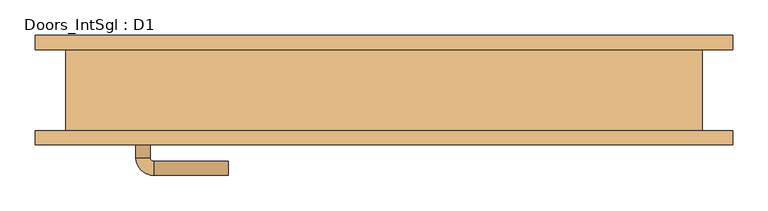
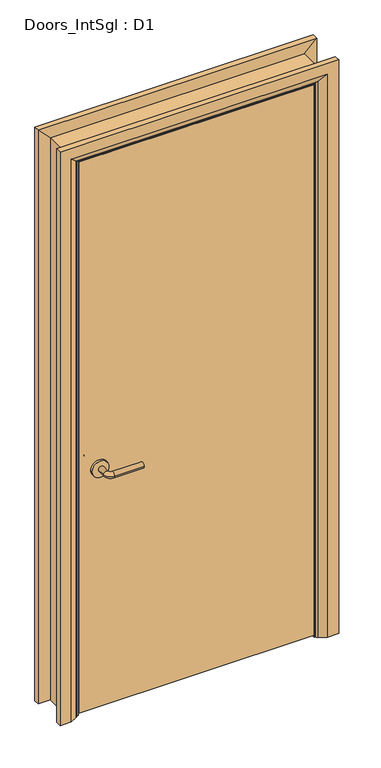
"""IFC4 building model written with IfcOpenShell, lengths in millimetres: door geometry, Doors_IntSgl : D1."""

from ifc_helpers import new_model, si_unit, point, frame, frame_2d, origin, place, context, project, spatial, polyline, circle_curve, ellipse_curve, trimmed, segment, composite_curve, outline, extrude, faceted_brep, source, transform, mapped, element, save
from ifc_brep_helpers import plane_surface, cylinder_surface, revolved_surface, advanced_brep


def doors_intsgl_d1_d2de26da(model_context):
    return source(origin(), model_context, "Body", "SolidModel", [
        advanced_brep(
        [(-350.2, -11.15, 900.0), (-330.2, -11.15, 900.0), (-350.2, 18.85, 900.0), (-330.2, 18.85, 900.0), (-325.2, 23.85, 900.0), (-325.2, 43.85, 900.0), (-220.2, 43.85, 900.0), (-220.2, 23.85, 900.0)],
        [
            (0, 1, circle_curve(frame((-340.2, -11.15, 900.0), z_axis=(0.0, -1.0, 0.0), x_axis=(1.0, 0.0, 0.0)), 10.0)),
            (1, 0, circle_curve(frame((-340.2, -11.15, 900.0), z_axis=(0.0, -1.0, 0.0), x_axis=(1.0, 0.0, 0.0)), 10.0)),
            (0, 2),
            (2, 3, circle_curve(frame((-340.2, 18.85, 900.0), z_axis=(0.0, -1.0, 0.0), x_axis=(1.0, 0.0, 0.0)), 10.0)),
            (3, 1),
            (3, 2, circle_curve(frame((-340.2, 18.85, 900.0), z_axis=(0.0, -1.0, 0.0), x_axis=(1.0, 0.0, 0.0)), 10.0)),
            (4, 3, circle_curve(frame((-325.2, 18.85, 900.0), z_axis=(0.0, 0.0, 1.0), x_axis=(-1.0, 0.0, 0.0)), 5.0)),
            (2, 5, circle_curve(frame((-325.2, 18.85, 900.0), z_axis=(0.0, 0.0, -1.0), x_axis=(-1.0, 0.0, 0.0)), 25.0)),
            (5, 4, circle_curve(frame((-325.2, 33.85, 900.0), z_axis=(-1.0, 0.0, 0.0), x_axis=(0.0, -1.0, 0.0)), 10.0)),
            (4, 5, circle_curve(frame((-325.2, 33.85, 900.0), z_axis=(-1.0, 0.0, 0.0), x_axis=(0.0, -1.0, 0.0)), 10.0)),
            (6, 7, circle_curve(frame((-220.2, 33.85, 900.0), z_axis=(1.0, 0.0, 0.0), x_axis=(0.0, -1.0, 0.0)), 10.0)),
            (7, 6, circle_curve(frame((-220.2, 33.85, 900.0), z_axis=(1.0, 0.0, 0.0), x_axis=(0.0, -1.0, 0.0)), 10.0)),
            (5, 6),
            (7, 4),
        ],
        [
            plane_surface(frame((-340.2, -11.15, 900.0), z_axis=(0.0, -1.0, 0.0), x_axis=(0.0, 0.0, 1.0))),
            cylinder_surface(frame((-340.2, -11.15, 900.0), z_axis=(0.0, -1.0, 0.0), x_axis=(1.0, 0.0, 0.0)), 10.0),
            revolved_surface(trimmed(ellipse_curve(frame((-340.2, 18.85, 900.0), z_axis=(0.0, -1.0, 0.0), x_axis=(1.0, 0.0, 0.0)), 10.0, 10.0), [point((-350.2, 18.85, 900.0))], [point((-330.2, 18.85, 900.0))], True, "CARTESIAN"), (-325.2, 18.85, 900.0), (0.0, 0.0, -1.0)),
            revolved_surface(trimmed(ellipse_curve(frame((-340.2, 18.85, 900.0), z_axis=(0.0, -1.0, 0.0), x_axis=(1.0, 0.0, 0.0)), 10.0, 10.0), [point((-330.2, 18.85, 900.0))], [point((-350.2, 18.85, 900.0))], True, "CARTESIAN"), (-325.2, 18.85, 900.0), (0.0, 0.0, -1.0)),
            plane_surface(frame((-220.2, 33.85, 900.0), z_axis=(1.0, 0.0, 0.0), x_axis=(0.0, 0.0, 1.0))),
            cylinder_surface(frame((-325.2, 33.85, 900.0), z_axis=(-1.0, 0.0, 0.0), x_axis=(0.0, -1.0, 0.0)), 10.0),
        ],
        [
            (0, [[1, 2]]),
            (1, [[-1, 3, 4, 5]]),
            (1, [[-2, -5, 6, -3]]),
            (2, [[7, -4, 8, 9]]),
            (3, [[-8, -6, -7, 10]]),
            (4, [[11, 12]]),
            (5, [[-9, 13, -12, 14]]),
            (5, [[-10, -14, -11, -13]]),
        ],
    ),
        extrude(outline(composite_curve([segment(trimmed(circle_curve(frame_2d((900.0, -342.7)), 30.0), [point((900.0, -372.7))], [point((900.0, -312.7))], False, "CARTESIAN"), True, "CONTINUOUS"), segment(trimmed(circle_curve(frame_2d((900.0, -342.7)), 30.0), [point((900.0, -312.7))], [point((900.0, -372.7))], False, "CARTESIAN"), True, "CONTINUOUS")], self_intersect=False)), frame((0.0, -19.15, 0.0), z_axis=(0.0, 1.0, 0.0), x_axis=(0.0, 0.0, 1.0)), (0.0, 0.0, 1.0), 8.0),
        advanced_brep(
        [(-350.2, -65.15, 900.0), (-330.2, -65.15, 900.0), (-330.2, -95.15, 900.0), (-350.2, -95.15, 900.0), (-325.2, -100.15, 900.0), (-325.2, -120.15, 900.0), (-220.2, -120.15, 900.0), (-220.2, -100.15, 900.0)],
        [
            (0, 1, circle_curve(frame((-340.2, -65.15, 900.0), z_axis=(0.0, 1.0, 0.0), x_axis=(1.0, 0.0, 0.0)), 10.0)),
            (1, 0, circle_curve(frame((-340.2, -65.15, 900.0), z_axis=(0.0, 1.0, 0.0), x_axis=(1.0, 0.0, 0.0)), 10.0)),
            (1, 2),
            (2, 3, circle_curve(frame((-340.2, -95.15, 900.0), z_axis=(0.0, 1.0, 0.0), x_axis=(1.0, 0.0, 0.0)), 10.0)),
            (3, 0),
            (3, 2, circle_curve(frame((-340.2, -95.15, 900.0), z_axis=(0.0, 1.0, 0.0), x_axis=(1.0, 0.0, 0.0)), 10.0)),
            (4, 5, circle_curve(frame((-325.2, -110.15, 900.0), z_axis=(-1.0, 0.0, 0.0), x_axis=(0.0, 1.0, 0.0)), 10.0)),
            (5, 3, circle_curve(frame((-325.2, -95.15, 900.0), z_axis=(0.0, 0.0, -1.0), x_axis=(-1.0, 0.0, 0.0)), 25.0)),
            (2, 4, circle_curve(frame((-325.2, -95.15, 900.0), z_axis=(0.0, 0.0, 1.0), x_axis=(-1.0, 0.0, 0.0)), 5.0)),
            (5, 4, circle_curve(frame((-325.2, -110.15, 900.0), z_axis=(-1.0, 0.0, 0.0), x_axis=(0.0, 1.0, 0.0)), 10.0)),
            (6, 7, circle_curve(frame((-220.2, -110.15, 900.0), z_axis=(1.0, 0.0, 0.0), x_axis=(0.0, 1.0, 0.0)), 10.0)),
            (7, 6, circle_curve(frame((-220.2, -110.15, 900.0), z_axis=(1.0, 0.0, 0.0), x_axis=(0.0, 1.0, 0.0)), 10.0)),
            (4, 7),
            (6, 5),
        ],
        [
            plane_surface(frame((-340.2, -65.15, 900.0), z_axis=(0.0, 1.0, 0.0), x_axis=(0.0, 0.0, 1.0))),
            cylinder_surface(frame((-340.2, -65.15, 900.0), z_axis=(0.0, 1.0, 0.0), x_axis=(1.0, 0.0, 0.0)), 10.0),
            revolved_surface(trimmed(ellipse_curve(frame((-340.2, -95.15, 900.0), z_axis=(0.0, -1.0, 0.0), x_axis=(1.0, 0.0, 0.0)), 10.0, 10.0), [point((-350.2, -95.15, 900.0))], [point((-330.2, -95.15, 900.0))], True, "CARTESIAN"), (-325.2, -95.15, 900.0), (0.0, 0.0, -1.0)),
            revolved_surface(trimmed(ellipse_curve(frame((-340.2, -95.15, 900.0), z_axis=(0.0, -1.0, 0.0), x_axis=(1.0, 0.0, 0.0)), 10.0, 10.0), [point((-330.2, -95.15, 900.0))], [point((-350.2, -95.15, 900.0))], True, "CARTESIAN"), (-325.2, -95.15, 900.0), (0.0, 0.0, -1.0)),
            plane_surface(frame((-220.2, -110.15, 900.0), z_axis=(1.0, 0.0, 0.0), x_axis=(0.0, 0.0, 1.0))),
            cylinder_surface(frame((-325.2, -110.15, 900.0), z_axis=(-1.0, 0.0, 0.0), x_axis=(0.0, 1.0, 0.0)), 10.0),
        ],
        [
            (0, [[1, 2]]),
            (1, [[3, 4, 5, -2]]),
            (1, [[-5, 6, -3, -1]]),
            (2, [[7, 8, -4, 9]]),
            (3, [[10, -9, -6, -8]]),
            (4, [[11, 12]]),
            (5, [[13, -11, 14, -7]]),
            (5, [[-14, -12, -13, -10]]),
        ],
    ),
        extrude(outline(composite_curve([segment(trimmed(circle_curve(frame_2d((900.0, -342.7)), 30.0), [point((900.0, -372.7))], [point((900.0, -312.7))], False, "CARTESIAN"), True, "CONTINUOUS"), segment(trimmed(circle_curve(frame_2d((900.0, -342.7)), 30.0), [point((900.0, -312.7))], [point((900.0, -372.7))], False, "CARTESIAN"), True, "CONTINUOUS")], self_intersect=False)), frame((0.0, -65.15, 0.0), z_axis=(0.0, 1.0, 0.0), x_axis=(0.0, 0.0, 1.0)), (0.0, 0.0, 1.0), 8.0),
        extrude(outline(polyline([(415.2, -19.15), (415.2, -57.15), (-415.2, -57.15), (-415.2, -19.15), (415.2, -19.15)])), frame((0.0, 0.0, 8.0), z_axis=(0.0, 0.0, 1.0), x_axis=(1.0, 0.0, 0.0)), (0.0, 0.0, 1.0), 2060.0),
        advanced_brep(
        [(492.2, -77.15, 0.0), (452.2, -77.15, 0.0), (426.2, -63.15, 0.0), (422.2, -57.15, 0.0), (492.2, -57.15, 0.0), (492.2, -57.15, 2145.0), (492.2, -77.15, 2145.0), (422.2, -57.15, 2075.0), (-422.2, -57.15, 2075.0), (-422.2, -57.15, 0.0), (-492.2, -57.15, 0.0), (-492.2, -57.15, 2145.0), (426.2, -63.15, 2079.0), (452.2, -77.15, 2105.0), (-492.2, -77.15, 2145.0), (-492.2, -77.15, 0.0), (-452.2, -77.15, 0.0), (-452.2, -77.15, 2105.0), (-426.2, -63.15, 0.0), (-426.2, -63.15, 2079.0)],
        [
            (0, 1),
            (1, 2),
            (2, 3, circle_curve(frame((430.2, -56.15, 0.0), z_axis=(0.0, 0.0, -1.0), x_axis=(1.0, 0.0, 0.0)), 8.0622577)),
            (3, 4),
            (4, 0),
            (4, 5),
            (5, 6),
            (6, 0),
            (3, 7),
            (7, 8),
            (8, 9),
            (9, 10),
            (10, 11),
            (11, 5),
            (2, 12),
            (12, 7, ellipse_curve(frame((430.2, -56.15, 2083.0), z_axis=(0.7071067811865475, 0.0, -0.7071067811865475), x_axis=(-0.7071067811865474, 0.0, -0.7071067811865476)), 11.4017543, 8.0622577)),
            (1, 13),
            (13, 12),
            (6, 14),
            (14, 15),
            (15, 16),
            (16, 17),
            (17, 13),
            (10, 15),
            (14, 11),
            (9, 18, circle_curve(frame((-430.2, -56.15, 0.0), z_axis=(0.0, 0.0, -1.0), x_axis=(-1.0, 0.0, 0.0)), 8.0622577)),
            (18, 16),
            (19, 18),
            (8, 19, ellipse_curve(frame((-430.2, -56.15, 2083.0), z_axis=(-0.7071067811865475, 0.0, -0.7071067811865475), x_axis=(-0.7071067811865474, 0.0, 0.7071067811865476)), 11.4017543, 8.0622577)),
            (19, 17),
            (12, 19),
        ],
        [
            plane_surface(frame((422.2, -57.15, 0.0), z_axis=(0.0, 0.0, -1.0), x_axis=(0.0, 1.0, 0.0))),
            plane_surface(frame((492.2, -77.15, 0.0), z_axis=(1.0, 0.0, 0.0), x_axis=(0.0, 0.0, 1.0))),
            plane_surface(frame((492.2, -57.15, 0.0), z_axis=(0.0, 1.0, 0.0), x_axis=(0.0, 0.0, 1.0))),
            cylinder_surface(frame((430.2, -56.15, 0.0), z_axis=(0.0, 0.0, -1.0), x_axis=(1.0, 0.0, 0.0)), 8.0622577),
            plane_surface(frame((426.2, -63.15, 0.0), z_axis=(-0.4740998230350126, -0.880471099922178, 0.0), x_axis=(0.0, 0.0, 1.0))),
            plane_surface(frame((452.2, -77.15, 0.0), z_axis=(0.0, -1.0, 0.0), x_axis=(0.0, 0.0, 1.0))),
            plane_surface(frame((-492.2, -77.15, 2145.0), z_axis=(-1.0, 0.0, 0.0), x_axis=(0.0, 0.0, -1.0))),
            plane_surface(frame((-422.2, -57.15, 0.0), z_axis=(0.0, 0.0, -1.0), x_axis=(0.0, 1.0, 0.0))),
            cylinder_surface(frame((-430.2, -56.15, 2075.0), z_axis=(0.0, 0.0, 1.0), x_axis=(-1.0, 0.0, 0.0)), 8.0622577),
            plane_surface(frame((-426.2, -63.15, 2079.0), z_axis=(0.47409982303501824, -0.8804710999221749, 0.0), x_axis=(0.0, 0.0, -1.0))),
            plane_surface(frame((492.2, -77.15, 2145.0), z_axis=(0.0, 0.0, 1.0), x_axis=(-1.0, 0.0, 0.0))),
            cylinder_surface(frame((422.2, -56.15, 2083.0), z_axis=(1.0, 0.0, 0.0), x_axis=(0.0, 0.0, 1.0)), 8.0622577),
            plane_surface(frame((426.2, -63.15, 2079.0), z_axis=(0.0, -0.8804710999221764, -0.4740998230350154), x_axis=(-1.0, 0.0, 0.0))),
        ],
        [
            (0, [[1, 2, 3, 4, 5]]),
            (1, [[6, 7, 8, -5]]),
            (2, [[9, 10, 11, 12, 13, 14, -6, -4]]),
            (3, [[15, 16, -9, -3]]),
            (4, [[17, 18, -15, -2]]),
            (5, [[-8, 19, 20, 21, 22, 23, -17, -1]]),
            (6, [[-13, 24, -20, 25]]),
            (7, [[-24, -12, 26, 27, -21]]),
            (8, [[28, -26, -11, 29]]),
            (9, [[-22, -27, -28, 30]]),
            (10, [[-14, -25, -19, -7]]),
            (11, [[31, -29, -10, -16]]),
            (12, [[-23, -30, -31, -18]]),
        ],
    ),
        extrude(outline(polyline([(0.0, -398.2), (2051.0, -398.2), (2051.0, 398.2), (0.0, 398.2), (0.0, 417.2), (2070.0, 417.2), (2070.0, -417.2), (0.0, -417.2), (0.0, -398.2)])), frame((0.0, -17.15, 0.0), z_axis=(0.0, 1.0, 0.0), x_axis=(0.0, 0.0, 1.0)), (0.0, 0.0, 1.0), 32.0),
        advanced_brep(
        [(-492.2, 77.15, 0.0), (-452.2, 77.15, 0.0), (-426.2, 63.15, 0.0), (-422.2, 57.15, 0.0), (-492.2, 57.15, 0.0), (-492.2, 57.15, 2145.0), (-492.2, 77.15, 2145.0), (-422.2, 57.15, 2075.0), (-426.2, 63.15, 2079.0), (-452.2, 77.15, 2105.0), (492.2, 77.15, 0.0), (492.2, 57.15, 0.0), (422.2, 57.15, 0.0), (426.2, 63.15, 0.0), (452.2, 77.15, 0.0), (492.2, 77.15, 2145.0), (452.2, 77.15, 2105.0), (426.2, 63.15, 2079.0), (422.2, 57.15, 2075.0), (492.2, 57.15, 2145.0)],
        [
            (0, 1),
            (1, 2),
            (2, 3, circle_curve(frame((-430.2, 56.15, 0.0), z_axis=(0.0, 0.0, -1.0), x_axis=(-1.0, 0.0, 0.0)), 8.0622577)),
            (3, 4),
            (4, 0),
            (4, 5),
            (5, 6),
            (6, 0),
            (3, 7),
            (7, 5),
            (2, 8),
            (8, 7, ellipse_curve(frame((-430.2, 56.15, 2083.0), z_axis=(-0.7071067811865475, 0.0, -0.7071067811865475), x_axis=(0.7071067811865474, 0.0, -0.7071067811865476)), 11.4017543, 8.0622577)),
            (1, 9),
            (9, 8),
            (6, 9),
            (10, 11),
            (11, 12),
            (12, 13, circle_curve(frame((430.2, 56.15, 0.0), z_axis=(0.0, 0.0, -1.0), x_axis=(1.0, 0.0, 0.0)), 8.0622577)),
            (13, 14),
            (14, 10),
            (15, 10),
            (14, 16),
            (16, 15),
            (13, 17),
            (17, 16),
            (12, 18),
            (18, 17, ellipse_curve(frame((430.2, 56.15, 2083.0), z_axis=(0.7071067811865475, 0.0, -0.7071067811865475), x_axis=(0.7071067811865474, 0.0, 0.7071067811865476)), 11.4017543, 8.0622577)),
            (11, 19),
            (19, 18),
            (15, 19),
            (5, 19),
            (15, 6),
            (7, 18),
            (8, 17),
            (9, 16),
        ],
        [
            plane_surface(frame((-422.2, 129.9510989, 0.0), z_axis=(0.0, 0.0, -1.0), x_axis=(1.0, 0.0, 0.0))),
            plane_surface(frame((-492.2, 77.15, 0.0), z_axis=(-1.0, 0.0, 0.0), x_axis=(0.0, 0.0, 1.0))),
            plane_surface(frame((-492.2, 57.15, 0.0), z_axis=(0.0, -1.0, 0.0), x_axis=(0.0, 0.0, 1.0))),
            cylinder_surface(frame((-430.2, 56.15, 0.0), z_axis=(0.0, 0.0, -1.0), x_axis=(-1.0, 0.0, 0.0)), 8.0622577),
            plane_surface(frame((-426.2, 63.15, 0.0), z_axis=(0.4740998230350183, 0.8804710999221749, 0.0), x_axis=(0.0, 0.0, 1.0))),
            plane_surface(frame((-452.2, 77.15, 0.0), z_axis=(0.0, 1.0, 0.0), x_axis=(0.0, 0.0, 1.0))),
            plane_surface(frame((422.2, 129.9510989, 0.0), z_axis=(0.0, 0.0, -1.0), x_axis=(-1.0, 0.0, 0.0))),
            plane_surface(frame((452.2, 77.15, 2105.0), z_axis=(0.0, 1.0, 0.0), x_axis=(0.0, 0.0, -1.0))),
            plane_surface(frame((426.2, 63.15, 2079.0), z_axis=(-0.4740998230350183, 0.8804710999221749, 0.0), x_axis=(0.0, 0.0, -1.0))),
            cylinder_surface(frame((430.2, 56.15, 2075.0), z_axis=(0.0, 0.0, 1.0), x_axis=(1.0, 0.0, 0.0)), 8.0622577),
            plane_surface(frame((492.2, 57.15, 2145.0), z_axis=(0.0, -1.0, 0.0), x_axis=(0.0, 0.0, -1.0))),
            plane_surface(frame((492.2, 77.15, 2145.0), z_axis=(1.0, 0.0, 0.0), x_axis=(0.0, 0.0, -1.0))),
            plane_surface(frame((-492.2, 77.15, 2145.0), z_axis=(0.0, 0.0, 1.0), x_axis=(1.0, 0.0, 0.0))),
            plane_surface(frame((-492.2, 57.15, 2145.0), z_axis=(0.0, -1.0, 0.0), x_axis=(1.0, 0.0, 0.0))),
            cylinder_surface(frame((-422.2, 56.15, 2083.0), z_axis=(-1.0, 0.0, 0.0), x_axis=(0.0, 0.0, 1.0)), 8.0622577),
            plane_surface(frame((-426.2, 63.15, 2079.0), z_axis=(0.0, 0.8804710999221749, -0.4740998230350183), x_axis=(1.0, 0.0, 0.0))),
            plane_surface(frame((-452.2, 77.15, 2105.0), z_axis=(0.0, 1.0, 0.0), x_axis=(1.0, 0.0, 0.0))),
        ],
        [
            (0, [[1, 2, 3, 4, 5]]),
            (1, [[6, 7, 8, -5]]),
            (2, [[9, 10, -6, -4]]),
            (3, [[11, 12, -9, -3]]),
            (4, [[13, 14, -11, -2]]),
            (5, [[-8, 15, -13, -1]]),
            (6, [[16, 17, 18, 19, 20]]),
            (7, [[21, -20, 22, 23]]),
            (8, [[-22, -19, 24, 25]]),
            (9, [[-24, -18, 26, 27]]),
            (10, [[-26, -17, 28, 29]]),
            (11, [[-28, -16, -21, 30]]),
            (12, [[31, -30, 32, -7]]),
            (13, [[33, -29, -31, -10]]),
            (14, [[34, -27, -33, -12]]),
            (15, [[35, -25, -34, -14]]),
            (16, [[-32, -23, -35, -15]]),
        ],
    ),
        faceted_brep([(-417.2, -57.15, 0.0), (-449.2, -57.15, 0.0), (-449.2, 57.15, 0.0), (-417.2, 57.15, 0.0), (-417.2, 57.15, 2070.0), (-417.2, -57.15, 2070.0), (-449.2, 57.15, 2102.0), (-449.2, -57.15, 2102.0), (417.2, -57.15, 0.0), (417.2, 57.15, 0.0), (449.2, 57.15, 0.0), (449.2, -57.15, 0.0), (417.2, -57.15, 2070.0), (449.2, -57.15, 2102.0), (449.2, 57.15, 2102.0), (417.2, 57.15, 2070.0)], [[[0, 1, 2, 3]], [[3, 4, 5, 0]], [[2, 6, 4, 3]], [[1, 7, 6, 2]], [[0, 5, 7, 1]], [[8, 9, 10, 11]], [[12, 8, 11, 13]], [[13, 11, 10, 14]], [[14, 10, 9, 15]], [[15, 9, 8, 12]], [[4, 15, 12, 5]], [[6, 14, 15, 4]], [[7, 13, 14, 6]], [[5, 12, 13, 7]]]),
    ])


if __name__ == "__main__":
    model = new_model("IFC4")
    model_context = context("Model", 3, world=origin())
    ifc_project = project(units=[si_unit("LENGTHUNIT", "METRE", prefix="MILLI")], contexts=[model_context])
    site = spatial("IfcSite", under=ifc_project)
    building = spatial("IfcBuilding", under=site)
    placement = place(None, origin())
    doors_intsgl_d1_shape = doors_intsgl_d1_d2de26da(model_context)
    element("IfcDoor", 1, ObjectType="Doors_IntSgl : D1", at=placement, inside=building, context=model_context, shape_type="MappedRepresentation", body=[
        mapped(doors_intsgl_d1_shape, transform((0.0, 0.0, 0.0), x_axis=(1.0, 0.0, 0.0), y_axis=(0.0, 1.0, 0.0), z_axis=(0.0, 0.0, 1.0))),
    ])
    save(model, "model.ifc")

# Revit data of these elements
# Type "Doors_IntSgl : D1"
#   Type Mark = "46"
#   Type Comments = "Internal Single"
#   Operation = "SingleSwingRight"
#   Manufacturer = "Revit"
#   Keynote = "L20"
#   Description = "Internal Single Door"
#   Analytic Construction = "Metal"
#   UnderCut = 0.026247 ft
#   Tolerance = 0.006562 ft
#   Thickness = 0.124672 ft
#   Thermal Resistance (R) = 0.270117 (m²·K)/W
#   Structural Tolerance = 0.026247 ft
#   StopDepth = 0.104987 ft
#   Stop Thickness = 0.062336 ft
#   Rough Width = 3.0 ft
#   Rough Height = 6.922572 ft
#   Height to Top Lock Rail = 3.28084 ft
#   Heat Transfer Coefficient (U) = 3.7021 W/(m²·K)
#   Handle Z Distance = 2.952756 ft
#   Handle X Distance = 0.246063 ft
#   Frame Thickness = 0.104987 ft
#   Door Panel Width = 2.724409 ft
#   Door Panel Thickness = 0.124672 ft
#   Door Panel Offset = 0.0 ft
#   Height = 6.922572 ft
#   Width = 3.0 ft
#   Door Panel Height = 6.75853 ft
#   Architrave Setback = 0.016404 ft
#   Vis - Ironmongery = yes
#   Material Ironmongery = Door - Handle
#   Material Frame = Door - Frame/Mullion (1)
#   Material Door = Door - Panel
#   Material Architrave = Door - Architrave
#   Visual Light Transmittance = 0
#   Solar Heat Gain Coefficient = 0
#   Function = (empty or 0)
#   Wall Closure = (empty or 0)
# Element 1 (IfcDoor, "Doors_IntSgl : D1")
#   Materials on its faces: "Door - Architrave", "Door - Handle", "Door - Frame/Mullion (1)", "Door - Panel"
# Materials
#   "Door - Handle": colour RGB 0 0 0, transparency 0, Keynote = "P21", Cost = 0
#   "Door - Frame/Mullion (1)": class "Wood", colour RGB 212 179 113, transparency 0, Keynote = "L20", Cost = 0
#   "Door - Panel": class "Wood", colour RGB 210 159 95, transparency 0, Keynote = "L20", Cost = 0
#   "Door - Architrave": class "Wood", colour RGB 154 90 5, transparency 0, Keynote = "P20", Cost = 0
